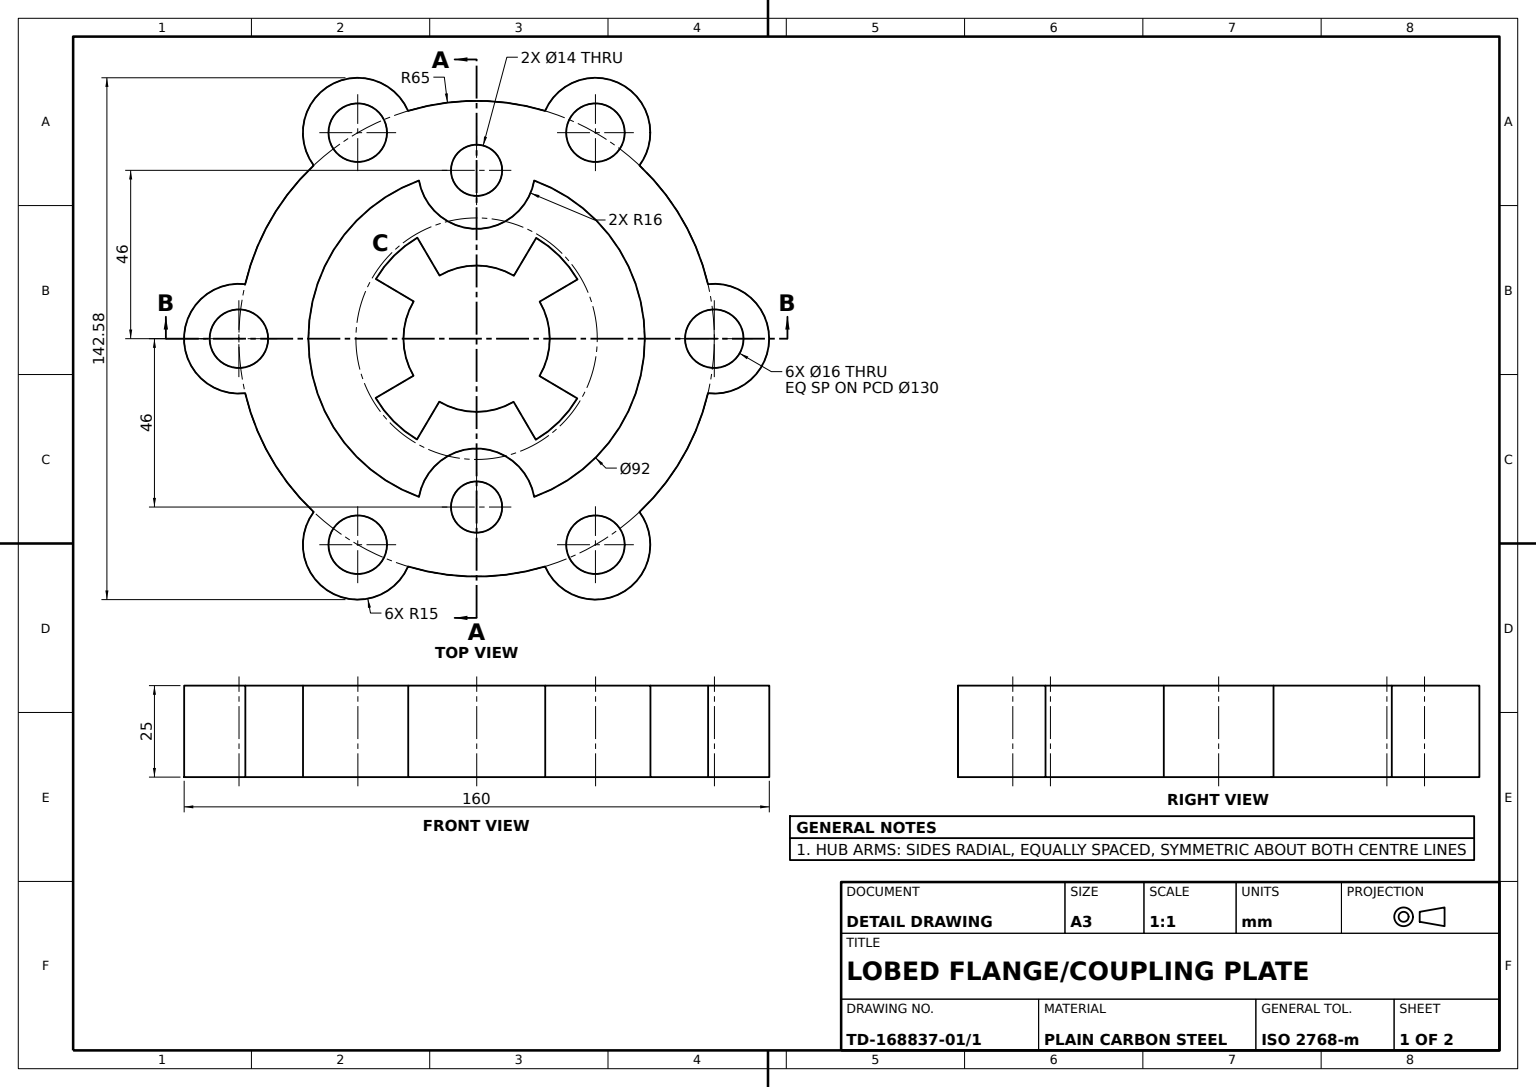
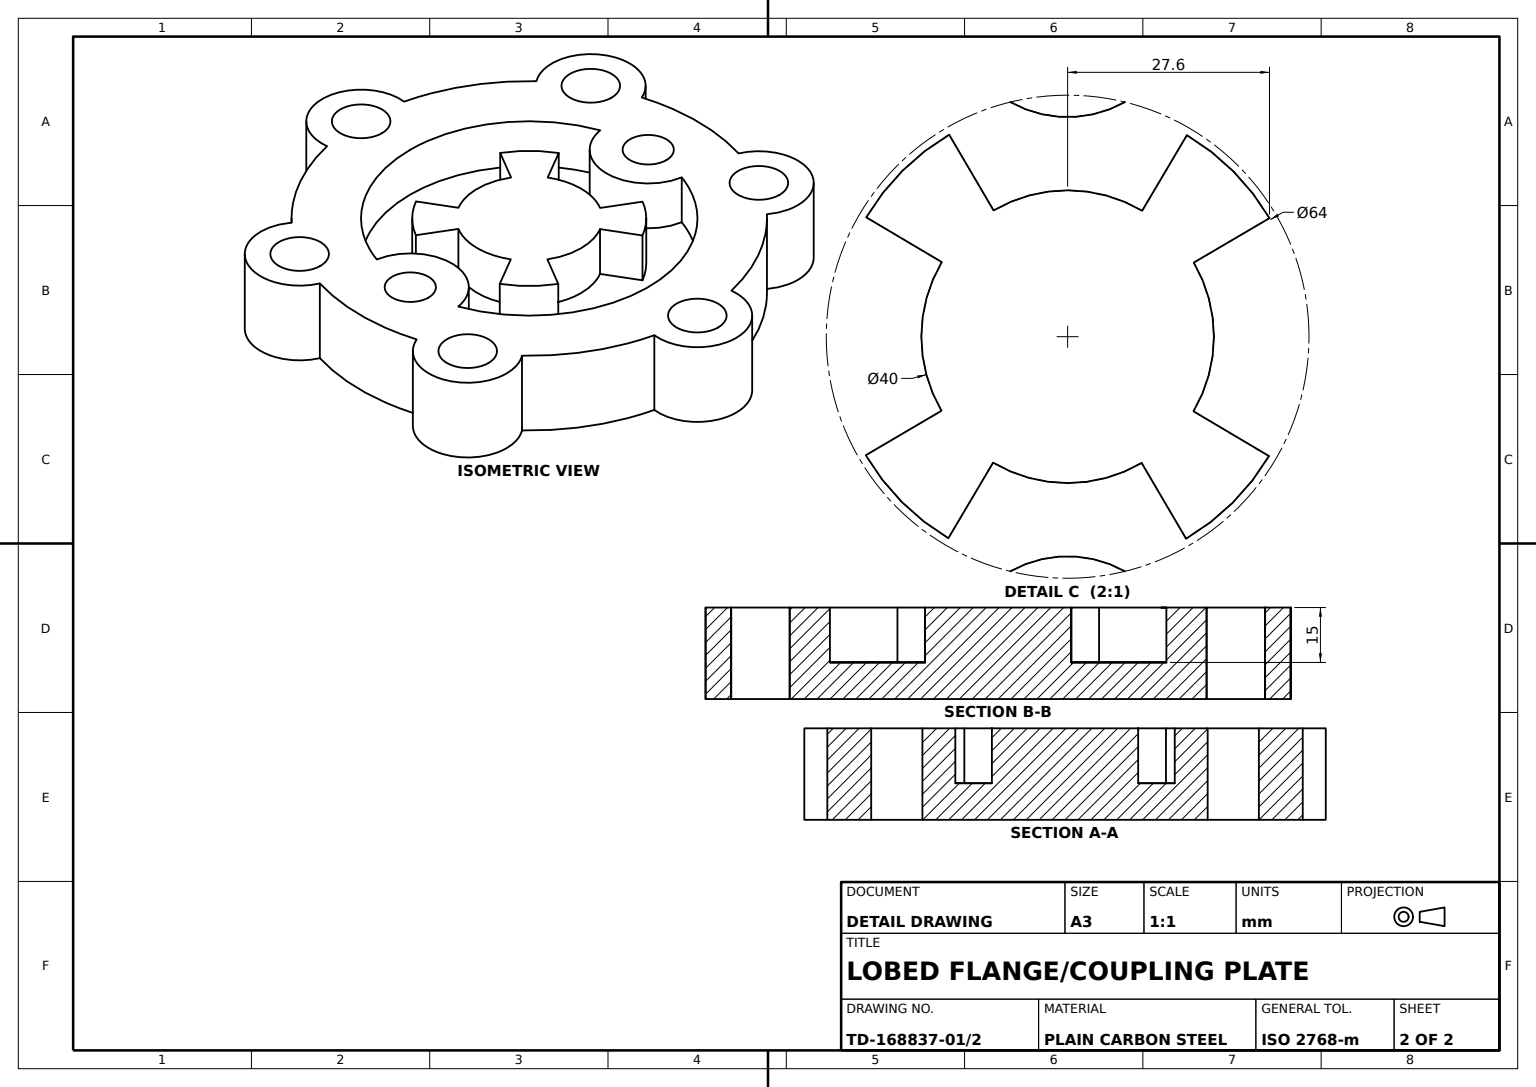
SolidWorks part; units mm, degrees
material "Plain Carbon Steel"
ref_plane "Front Plane" through (0, 0, 0) normal (0, 0, 1) x (1, 0, 0)
ref_plane "Top Plane" through (0, 0, 0) normal (0, 1, 0) x (1, 0, 0)
ref_plane "Right Plane" through (0, 0, 0) normal (1, 0, 0) x (0, 0, -1)
sketch "Flange Profile Sketch" plane through (0, 0, 0) normal (0, 1, 0) x (1, 0, 0)
  arc A0 (-14.8998, 63.2692) -> (-47.3429, 44.5382) centre (0, 0) ccw
  arc A1 (14.8998, 63.2692) -> (-14.8998, 63.2692) centre (0, 65) ccw
  arc A2 (62.2427, 18.731) -> (47.3429, 44.5382) centre (56.2917, 32.5) ccw
  arc A3 (47.3429, -44.5382) -> (62.2427, -18.731) centre (56.2917, -32.5) ccw
  arc A4 (-14.8998, -63.2692) -> (14.8998, -63.2692) centre (0, -65) ccw
  arc A5 (-62.2427, -18.731) -> (-47.3429, -44.5382) centre (-56.2917, -32.5) ccw
  arc A6 (-47.3429, 44.5382) -> (-62.2427, 18.731) centre (-56.2917, 32.5) ccw
  arc A7 (47.3429, 44.5382) -> (14.8998, 63.2692) centre (0, 0) ccw
  arc A8 (62.2427, -18.731) -> (62.2427, 18.731) centre (0, 0) ccw
  arc A9 (14.8998, -63.2692) -> (47.3429, -44.5382) centre (0, 0) ccw
  arc A10 (-47.3429, -44.5382) -> (-14.8998, -63.2692) centre (0, 0) ccw
  arc A11 (-62.2427, 18.731) -> (-62.2427, -18.731) centre (0, 0) ccw
  dimension "D1" = 130
  dimension "D2" = 30
  dimension "D3" = 6
  dimension "D4" = 56.2917
  dimension "D5" = 32.5
extrude "Flange Plate" add sketch "Flange Profile Sketch" along normal blind 25
sketch "Bolt Holes Sketch" plane through (0, 25, 0) normal (0, 1, 0) x (1, 0, 0)
  circle A0 centre (0, 65) radius 8
  circle A1 centre (56.2917, 32.5) radius 8
  circle A2 centre (56.2917, -32.5) radius 8
  circle A3 centre (0, -65) radius 8
  circle A4 centre (-56.2917, -32.5) radius 8
  circle A5 centre (-56.2917, 32.5) radius 8
  dimension "D1" = 16
  dimension "D3" = 56.2917
  dimension "D4" = 65
  dimension "D2" = 6
extrude "Bolt Holes 6xØ16" cut sketch "Bolt Holes Sketch" against normal blind 25
sketch "Recess Sketch" plane through (0, 25, 0) normal (0, 1, 0) x (1, 0, 0)
  arc A0 (-43.2174, -15.7562) -> (43.2174, -15.7562) centre (0, 0) ccw
  arc A1 (-43.2174, -15.7562) -> (-43.2174, 15.7562) centre (-46, 0) ccw
  arc A2 (43.2174, 15.7562) -> (43.2174, -15.7562) centre (46, 0) ccw
  arc A3 (43.2174, 15.7562) -> (-43.2174, 15.7562) centre (0, 0) ccw
  dimension "D1" = 92
  dimension "D2" = 32
  dimension "D3" = 32
extrude "Annular Recess Ø92" cut sketch "Recess Sketch" against normal blind 15
sketch "Lug Holes Sketch" plane through (0, 25, 0) normal (0, 1, 0) x (1, 0, 0)
  circle A0 centre (-46, 0) radius 7
  circle A1 centre (46, 0) radius 7
  dimension "D1" = 14
  dimension "D2" = 14
extrude "Lug Holes 2xØ14" cut sketch "Lug Holes Sketch" against normal through all
sketch "Centre Hub Sketch" plane through (0, 10, 0) normal (0, 1, 0) x (1, 0, 0)
  line L0 (17.208, -10.1924) -> (27.5328, -16.3078)
  line L1 (10.1924, 17.208) -> (16.3078, 27.5328)
  line L2 (17.2491, 10.1226) -> (27.5986, 16.1962)
  line L3 (10.1226, -17.2491) -> (16.1962, -27.5986)
  line L4 (-10.1924, -17.208) -> (-16.3078, -27.5328)
  line L5 (-17.2491, -10.1226) -> (-27.5986, -16.1962)
  line L6 (-17.208, 10.1924) -> (-27.5328, 16.3078)
  line L7 (-10.1226, 17.2491) -> (-16.1962, 27.5986)
  arc A0 (10.1924, 17.208) -> (-10.1226, 17.2491) centre (0, 0) ccw
  arc A1 (-16.1962, 27.5986) -> (-27.5328, 16.3078) centre (0, 0) ccw
  arc A2 (-17.208, 10.1924) -> (-17.2491, -10.1226) centre (0, 0) ccw
  arc A3 (-27.5986, -16.1962) -> (-16.3078, -27.5328) centre (0, 0) ccw
  arc A4 (-10.1924, -17.208) -> (10.1226, -17.2491) centre (0, 0) ccw
  arc A5 (16.1962, -27.5986) -> (27.5328, -16.3078) centre (0, 0) ccw
  arc A6 (17.208, -10.1924) -> (17.2491, 10.1226) centre (0, 0) ccw
  arc A7 (27.5986, 16.1962) -> (16.3078, 27.5328) centre (0, 0) ccw
  dimension "D1" = 40
  dimension "D2" = 64
  dimension "D3" = 16
  dimension "D4" = 10.1924
  dimension "D5" = 27.5986
  dimension "D6" = 10.1226
  dimension "D7" = 4
extrude "Keyed Centre Hub Ø40" add sketch "Centre Hub Sketch" along normal blind 15
